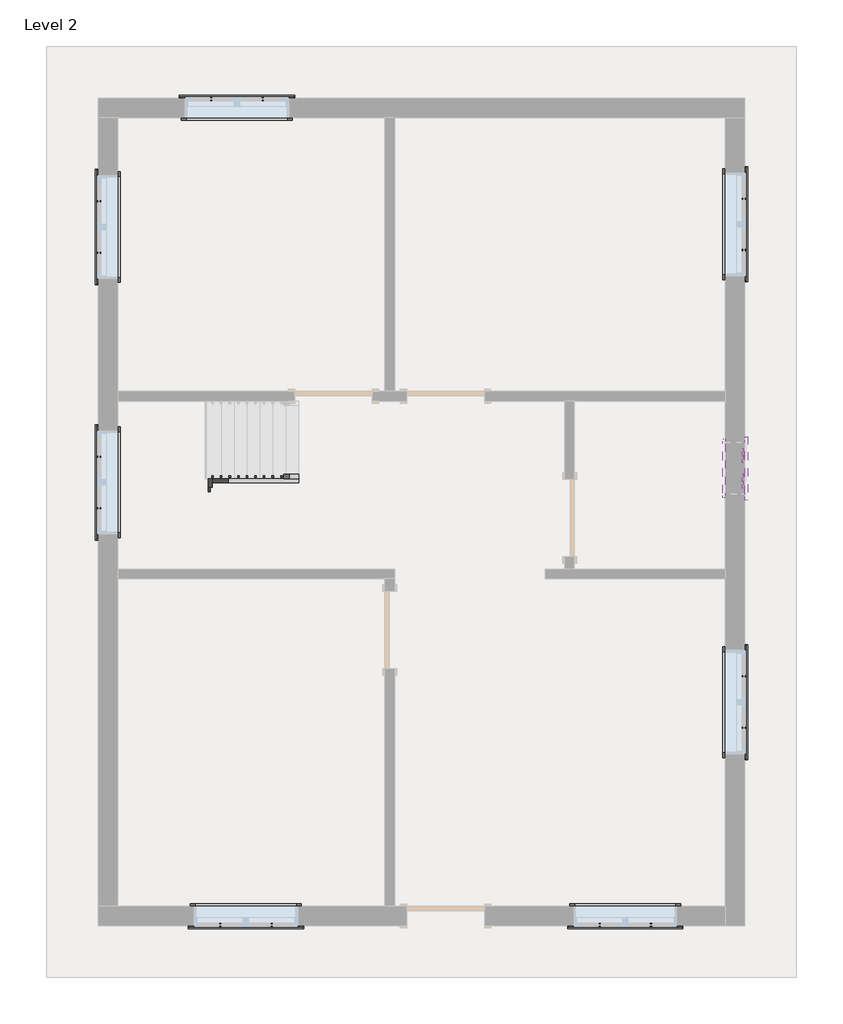
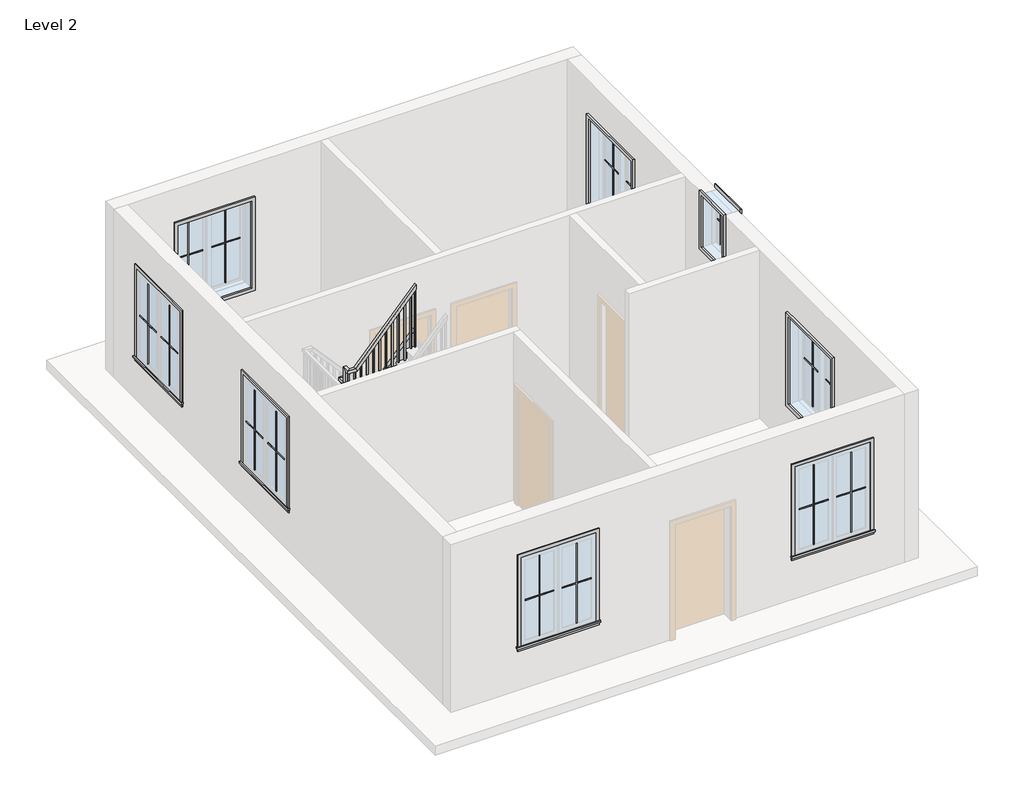
# One storey, part 2 of 2: 32 proxies, 3 members, 1 railing.
"""IFC4 building model written with IfcOpenShell, lengths in millimetres."""

from ifc_helpers import new_model, si_unit, frame, origin, place, context, project, spatial, polyline, outline, extrude, faceted_brep, transform, mapped, element, save
from components import muntin_pattern_2x2_muntin_pattern_2x2_6dad3731, muntin_pattern_2x2_muntin_pattern_2x2_a30a3345, muntin_pattern_2x2_muntin_pattern_2x2_53152e2c, muntin_pattern_2x2_muntin_pattern_2x2_e8f3e573, trim_window_exterior_flat_with_sill_92b9b949, trim_window_exterior_flat_with_sill_a665a915, trim_window_interior_flat_picture_frame_3bb882cf, trim_window_interior_flat_picture_frame_d485c387

model = new_model("IFC4")

# Units and contexts
model_context = context("Model", 3, world=origin())
ifc_project = project(units=[si_unit("LENGTHUNIT", "METRE", prefix="MILLI")], contexts=[model_context])

# Site, building, storey
site = spatial("IfcSite", under=ifc_project)
building = spatial("IfcBuilding", under=site)
storey = spatial("IfcBuildingStorey", under=building, Name="Level 2", Elevation=3048.0)

# Proxies
placement = place(None, origin())
muntin_pattern_2x2_muntin_pattern_2x2_shape = muntin_pattern_2x2_muntin_pattern_2x2_6dad3731(model_context)
element("IfcBuildingElementProxy", 1, Name="Muntin Pattern_2x2 : Muntin Pattern_2x2", ObjectType="Muntin Pattern_2x2 : Muntin Pattern_2x2", at=placement, inside=storey, context=model_context, shape_type="MappedRepresentation", body=[
    mapped(muntin_pattern_2x2_muntin_pattern_2x2_shape, transform((7785.1, 4733.925, 4032.25), x_axis=(-1.0, 0.0, 0.0), y_axis=(0.0, -1.0, 0.0), z_axis=(0.0, 0.0, 1.0))),
])
element("IfcBuildingElementProxy", 2, Name="Muntin Pattern_2x2 : Muntin Pattern_2x2", ObjectType="Muntin Pattern_2x2 : Muntin Pattern_2x2", at=placement, inside=storey, context=model_context, shape_type="MappedRepresentation", body=[
    mapped(muntin_pattern_2x2_muntin_pattern_2x2_shape, transform((3313.1125, 4733.925, 4032.25), x_axis=(-1.0, 0.0, 0.0), y_axis=(0.0, -1.0, 0.0), z_axis=(0.0, 0.0, 1.0))),
])
element("IfcBuildingElementProxy", 3, Name="Muntin Pattern_2x2 : Muntin Pattern_2x2", ObjectType="Muntin Pattern_2x2 : Muntin Pattern_2x2", at=placement, inside=storey, context=model_context, shape_type="MappedRepresentation", body=[
    mapped(muntin_pattern_2x2_muntin_pattern_2x2_shape, transform((8880.475, 13295.3125, 4032.25), x_axis=(0.0, -1.0, 0.0), y_axis=(1.0, 0.0, 0.0), z_axis=(0.0, 0.0, 1.0))),
])
element("IfcBuildingElementProxy", 4, Name="Muntin Pattern_2x2 : Muntin Pattern_2x2", ObjectType="Muntin Pattern_2x2 : Muntin Pattern_2x2", at=placement, inside=storey, context=model_context, shape_type="MappedRepresentation", body=[
    mapped(muntin_pattern_2x2_muntin_pattern_2x2_shape, transform((8880.475, 7662.8625, 4032.25), x_axis=(0.0, -1.0, 0.0), y_axis=(1.0, 0.0, 0.0), z_axis=(0.0, 0.0, 1.0))),
])
element("IfcBuildingElementProxy", 5, Name="Muntin Pattern_2x2 : Muntin Pattern_2x2", ObjectType="Muntin Pattern_2x2 : Muntin Pattern_2x2", at=placement, inside=storey, context=model_context, shape_type="MappedRepresentation", body=[
    mapped(muntin_pattern_2x2_muntin_pattern_2x2_shape, transform((1279.525, 12657.1375, 4032.25), x_axis=(0.0, 1.0, 0.0), y_axis=(-1.0, 0.0, 0.0), z_axis=(0.0, 0.0, 1.0))),
])
element("IfcBuildingElementProxy", 6, Name="Muntin Pattern_2x2 : Muntin Pattern_2x2", ObjectType="Muntin Pattern_2x2 : Muntin Pattern_2x2", at=placement, inside=storey, context=model_context, shape_type="MappedRepresentation", body=[
    mapped(muntin_pattern_2x2_muntin_pattern_2x2_shape, transform((1279.525, 9647.2375, 4032.25), x_axis=(0.0, 1.0, 0.0), y_axis=(-1.0, 0.0, 0.0), z_axis=(0.0, 0.0, 1.0))),
])
element("IfcBuildingElementProxy", 7, Name="Muntin Pattern_2x2 : Muntin Pattern_2x2", ObjectType="Muntin Pattern_2x2 : Muntin Pattern_2x2", at=placement, inside=storey, context=model_context, shape_type="MappedRepresentation", body=[
    mapped(muntin_pattern_2x2_muntin_pattern_2x2_shape, transform((2601.9125, 14468.475, 4032.25), x_axis=(1.0, 0.0, 0.0), y_axis=(0.0, 1.0, 0.0), z_axis=(0.0, 0.0, 1.0))),
])
muntin_pattern_2x2_muntin_pattern_2x2_2_shape = muntin_pattern_2x2_muntin_pattern_2x2_a30a3345(model_context)
element("IfcBuildingElementProxy", 8, Name="Muntin Pattern_2x2 : Muntin Pattern_2x2", ObjectType="Muntin Pattern_2x2 : Muntin Pattern_2x2", at=placement, inside=storey, context=model_context, shape_type="MappedRepresentation", body=[
    mapped(muntin_pattern_2x2_muntin_pattern_2x2_2_shape, transform((7178.675, 4733.925, 4032.25), x_axis=(1.0, 0.0, 0.0), y_axis=(0.0, 1.0, 0.0), z_axis=(0.0, 0.0, 1.0))),
])
element("IfcBuildingElementProxy", 9, Name="Muntin Pattern_2x2 : Muntin Pattern_2x2", ObjectType="Muntin Pattern_2x2 : Muntin Pattern_2x2", at=placement, inside=storey, context=model_context, shape_type="MappedRepresentation", body=[
    mapped(muntin_pattern_2x2_muntin_pattern_2x2_2_shape, transform((2706.6875, 4733.925, 4032.25), x_axis=(1.0, 0.0, 0.0), y_axis=(0.0, 1.0, 0.0), z_axis=(0.0, 0.0, 1.0))),
])
element("IfcBuildingElementProxy", 10, Name="Muntin Pattern_2x2 : Muntin Pattern_2x2", ObjectType="Muntin Pattern_2x2 : Muntin Pattern_2x2", at=placement, inside=storey, context=model_context, shape_type="MappedRepresentation", body=[
    mapped(muntin_pattern_2x2_muntin_pattern_2x2_2_shape, transform((8880.475, 12688.8875, 4032.25), x_axis=(0.0, 1.0, 0.0), y_axis=(-1.0, 0.0, 0.0), z_axis=(0.0, 0.0, 1.0))),
])
element("IfcBuildingElementProxy", 11, Name="Muntin Pattern_2x2 : Muntin Pattern_2x2", ObjectType="Muntin Pattern_2x2 : Muntin Pattern_2x2", at=placement, inside=storey, context=model_context, shape_type="MappedRepresentation", body=[
    mapped(muntin_pattern_2x2_muntin_pattern_2x2_2_shape, transform((8880.475, 7056.4375, 4032.25), x_axis=(0.0, 1.0, 0.0), y_axis=(-1.0, 0.0, 0.0), z_axis=(0.0, 0.0, 1.0))),
])
element("IfcBuildingElementProxy", 12, Name="Muntin Pattern_2x2 : Muntin Pattern_2x2", ObjectType="Muntin Pattern_2x2 : Muntin Pattern_2x2", at=placement, inside=storey, context=model_context, shape_type="MappedRepresentation", body=[
    mapped(muntin_pattern_2x2_muntin_pattern_2x2_2_shape, transform((1279.525, 13263.5625, 4032.25), x_axis=(0.0, -1.0, 0.0), y_axis=(1.0, 0.0, 0.0), z_axis=(0.0, 0.0, 1.0))),
])
element("IfcBuildingElementProxy", 13, Name="Muntin Pattern_2x2 : Muntin Pattern_2x2", ObjectType="Muntin Pattern_2x2 : Muntin Pattern_2x2", at=placement, inside=storey, context=model_context, shape_type="MappedRepresentation", body=[
    mapped(muntin_pattern_2x2_muntin_pattern_2x2_2_shape, transform((1279.525, 10253.6625, 4032.25), x_axis=(0.0, -1.0, 0.0), y_axis=(1.0, 0.0, 0.0), z_axis=(0.0, 0.0, 1.0))),
])
element("IfcBuildingElementProxy", 14, Name="Muntin Pattern_2x2 : Muntin Pattern_2x2", ObjectType="Muntin Pattern_2x2 : Muntin Pattern_2x2", at=placement, inside=storey, context=model_context, shape_type="MappedRepresentation", body=[
    mapped(muntin_pattern_2x2_muntin_pattern_2x2_2_shape, transform((3208.3375, 14468.475, 4032.25), x_axis=(-1.0, 0.0, 0.0), y_axis=(0.0, -1.0, 0.0), z_axis=(0.0, 0.0, 1.0))),
])
muntin_pattern_2x2_muntin_pattern_2x2_3_shape = muntin_pattern_2x2_muntin_pattern_2x2_53152e2c(model_context)
element("IfcBuildingElementProxy", 15, Name="Muntin Pattern_2x2 : Muntin Pattern_2x2", ObjectType="Muntin Pattern_2x2 : Muntin Pattern_2x2", at=placement, inside=storey, context=model_context, shape_type="MappedRepresentation", body=[
    mapped(muntin_pattern_2x2_muntin_pattern_2x2_3_shape, transform((8880.475, 10266.3625, 5251.45), x_axis=(0.0, -1.0, 0.0), y_axis=(1.0, 0.0, 0.0), z_axis=(0.0, 0.0, 1.0))),
])
muntin_pattern_2x2_muntin_pattern_2x2_4_shape = muntin_pattern_2x2_muntin_pattern_2x2_e8f3e573(model_context)
element("IfcBuildingElementProxy", 16, Name="Muntin Pattern_2x2 : Muntin Pattern_2x2", ObjectType="Muntin Pattern_2x2 : Muntin Pattern_2x2", at=placement, inside=storey, context=model_context, shape_type="MappedRepresentation", body=[
    mapped(muntin_pattern_2x2_muntin_pattern_2x2_4_shape, transform((8880.475, 9964.7375, 5251.45), x_axis=(0.0, 1.0, 0.0), y_axis=(-1.0, 0.0, 0.0), z_axis=(0.0, 0.0, 1.0))),
])
trim_window_exterior_flat_with_sill_shape = trim_window_exterior_flat_with_sill_92b9b949(model_context)
element("IfcBuildingElementProxy", 17, Name="Trim-Window-Exterior-Flat : with Sill", ObjectType="Trim-Window-Exterior-Flat : with Sill", at=placement, inside=storey, context=model_context, shape_type="MappedRepresentation", body=[
    mapped(trim_window_exterior_flat_with_sill_shape, transform((7481.8875, 4724.4, 5486.4), x_axis=(1.0, 0.0, 0.0), y_axis=(0.0, 0.0, 1.0), z_axis=(0.0, -1.0, 0.0))),
])
element("IfcBuildingElementProxy", 18, Name="Trim-Window-Exterior-Flat : with Sill", ObjectType="Trim-Window-Exterior-Flat : with Sill", at=placement, inside=storey, context=model_context, shape_type="MappedRepresentation", body=[
    mapped(trim_window_exterior_flat_with_sill_shape, transform((3009.9, 4724.4, 5486.4), x_axis=(1.0, 0.0, 0.0), y_axis=(0.0, 0.0, 1.0), z_axis=(0.0, -1.0, 0.0))),
])
element("IfcBuildingElementProxy", 19, Name="Trim-Window-Exterior-Flat : with Sill", ObjectType="Trim-Window-Exterior-Flat : with Sill", at=placement, inside=storey, context=model_context, shape_type="MappedRepresentation", body=[
    mapped(trim_window_exterior_flat_with_sill_shape, transform((8890.0, 12992.1, 5486.4), x_axis=(0.0, 1.0, 0.0), y_axis=(0.0, 0.0, 1.0), z_axis=(1.0, 0.0, 0.0))),
])
element("IfcBuildingElementProxy", 20, Name="Trim-Window-Exterior-Flat : with Sill", ObjectType="Trim-Window-Exterior-Flat : with Sill", at=placement, inside=storey, context=model_context, shape_type="MappedRepresentation", body=[
    mapped(trim_window_exterior_flat_with_sill_shape, transform((8890.0, 7359.65, 5486.4), x_axis=(0.0, 1.0, 0.0), y_axis=(0.0, 0.0, 1.0), z_axis=(1.0, 0.0, 0.0))),
])
element("IfcBuildingElementProxy", 21, Name="Trim-Window-Exterior-Flat : with Sill", ObjectType="Trim-Window-Exterior-Flat : with Sill", at=placement, inside=storey, context=model_context, shape_type="MappedRepresentation", body=[
    mapped(trim_window_exterior_flat_with_sill_shape, transform((1270.0, 12960.35, 5486.4), x_axis=(0.0, -1.0, 0.0), y_axis=(0.0, 0.0, 1.0), z_axis=(-1.0, 0.0, 0.0))),
])
element("IfcBuildingElementProxy", 22, Name="Trim-Window-Exterior-Flat : with Sill", ObjectType="Trim-Window-Exterior-Flat : with Sill", at=placement, inside=storey, context=model_context, shape_type="MappedRepresentation", body=[
    mapped(trim_window_exterior_flat_with_sill_shape, transform((1270.0, 9950.45, 5486.4), x_axis=(0.0, -1.0, 0.0), y_axis=(0.0, 0.0, 1.0), z_axis=(-1.0, 0.0, 0.0))),
])
element("IfcBuildingElementProxy", 23, Name="Trim-Window-Exterior-Flat : with Sill", ObjectType="Trim-Window-Exterior-Flat : with Sill", at=placement, inside=storey, context=model_context, shape_type="MappedRepresentation", body=[
    mapped(trim_window_exterior_flat_with_sill_shape, transform((2905.125, 14478.0, 5486.4), x_axis=(-1.0, 0.0, 0.0), y_axis=(0.0, 0.0, 1.0), z_axis=(0.0, 1.0, 0.0))),
])
trim_window_exterior_flat_with_sill_2_shape = trim_window_exterior_flat_with_sill_a665a915(model_context)
element("IfcBuildingElementProxy", 24, Name="Trim-Window-Exterior-Flat : with Sill", ObjectType="Trim-Window-Exterior-Flat : with Sill", at=placement, inside=storey, context=model_context, shape_type="MappedRepresentation", body=[
    mapped(trim_window_exterior_flat_with_sill_2_shape, transform((8890.0, 10115.55, 6096.0), x_axis=(0.0, 1.0, 0.0), y_axis=(0.0, 0.0, 1.0), z_axis=(1.0, 0.0, 0.0))),
])
trim_window_interior_flat_picture_frame_shape = trim_window_interior_flat_picture_frame_3bb882cf(model_context)
element("IfcBuildingElementProxy", 25, Name="Trim-Window-Interior-Flat : Picture Frame", ObjectType="Trim-Window-Interior-Flat : Picture Frame", at=placement, inside=storey, context=model_context, shape_type="MappedRepresentation", body=[
    mapped(trim_window_interior_flat_picture_frame_shape, transform((7481.8875, 4953.0, 5486.4), x_axis=(-1.0, 0.0, 0.0), y_axis=(0.0, 0.0, 1.0), z_axis=(0.0, 1.0, 0.0))),
])
element("IfcBuildingElementProxy", 26, Name="Trim-Window-Interior-Flat : Picture Frame", ObjectType="Trim-Window-Interior-Flat : Picture Frame", at=placement, inside=storey, context=model_context, shape_type="MappedRepresentation", body=[
    mapped(trim_window_interior_flat_picture_frame_shape, transform((3009.9, 4953.0, 5486.4), x_axis=(-1.0, 0.0, 0.0), y_axis=(0.0, 0.0, 1.0), z_axis=(0.0, 1.0, 0.0))),
])
element("IfcBuildingElementProxy", 27, Name="Trim-Window-Interior-Flat : Picture Frame", ObjectType="Trim-Window-Interior-Flat : Picture Frame", at=placement, inside=storey, context=model_context, shape_type="MappedRepresentation", body=[
    mapped(trim_window_interior_flat_picture_frame_shape, transform((8661.4, 12992.1, 5486.4), x_axis=(0.0, -1.0, 0.0), y_axis=(0.0, 0.0, 1.0), z_axis=(-1.0, 0.0, 0.0))),
])
element("IfcBuildingElementProxy", 28, Name="Trim-Window-Interior-Flat : Picture Frame", ObjectType="Trim-Window-Interior-Flat : Picture Frame", at=placement, inside=storey, context=model_context, shape_type="MappedRepresentation", body=[
    mapped(trim_window_interior_flat_picture_frame_shape, transform((8661.4, 7359.65, 5486.4), x_axis=(0.0, -1.0, 0.0), y_axis=(0.0, 0.0, 1.0), z_axis=(-1.0, 0.0, 0.0))),
])
element("IfcBuildingElementProxy", 29, Name="Trim-Window-Interior-Flat : Picture Frame", ObjectType="Trim-Window-Interior-Flat : Picture Frame", at=placement, inside=storey, context=model_context, shape_type="MappedRepresentation", body=[
    mapped(trim_window_interior_flat_picture_frame_shape, transform((1498.6, 12960.35, 5486.4), x_axis=(0.0, 1.0, 0.0), y_axis=(0.0, 0.0, 1.0), z_axis=(1.0, 0.0, 0.0))),
])
element("IfcBuildingElementProxy", 30, Name="Trim-Window-Interior-Flat : Picture Frame", ObjectType="Trim-Window-Interior-Flat : Picture Frame", at=placement, inside=storey, context=model_context, shape_type="MappedRepresentation", body=[
    mapped(trim_window_interior_flat_picture_frame_shape, transform((1498.6, 9950.45, 5486.4), x_axis=(0.0, 1.0, 0.0), y_axis=(0.0, 0.0, 1.0), z_axis=(1.0, 0.0, 0.0))),
])
element("IfcBuildingElementProxy", 31, Name="Trim-Window-Interior-Flat : Picture Frame", ObjectType="Trim-Window-Interior-Flat : Picture Frame", at=placement, inside=storey, context=model_context, shape_type="MappedRepresentation", body=[
    mapped(trim_window_interior_flat_picture_frame_shape, transform((2905.125, 14249.4, 5486.4), x_axis=(1.0, 0.0, 0.0), y_axis=(0.0, 0.0, 1.0), z_axis=(0.0, -1.0, 0.0))),
])
trim_window_interior_flat_picture_frame_2_shape = trim_window_interior_flat_picture_frame_d485c387(model_context)
element("IfcBuildingElementProxy", 32, Name="Trim-Window-Interior-Flat : Picture Frame", ObjectType="Trim-Window-Interior-Flat : Picture Frame", at=placement, inside=storey, context=model_context, shape_type="MappedRepresentation", body=[
    mapped(trim_window_interior_flat_picture_frame_2_shape, transform((8661.4, 10115.55, 6096.0), x_axis=(0.0, -1.0, 0.0), y_axis=(0.0, 0.0, 1.0), z_axis=(-1.0, 0.0, 0.0))),
])

# Members
element("IfcMember", 33, ObjectType="Stringer - 2\" Width", at=placement, inside=storey, context=model_context, shape_type="SweptSolid", body=[
    extrude(outline(polyline([(3048.0, 3632.2), (3322.6288314, 3632.2), (4451.5177203, 2616.2), (3995.8883192, 2616.2), (3048.0, 3469.2994873), (3048.0, 3632.2)])), frame((0.0, 9944.1, 0.0), z_axis=(0.0, 1.0, 0.0), x_axis=(0.0, 0.0, 1.0)), (0.0, 0.0, 1.0), 50.8),
])
element("IfcMember", 34, ObjectType="Stringer - 2\" Width", at=placement, inside=storey, context=model_context, shape_type="SweptSolid", body=[
    extrude(outline(polyline([(2565.4, 9994.9), (2616.2, 9994.9), (2616.2, 9893.3), (2565.4, 9893.3), (2565.4, 9994.9)])), frame((0.0, 0.0, 4174.0666667), z_axis=(0.0, 0.0, 1.0), x_axis=(1.0, 0.0, 0.0)), (0.0, 0.0, 1.0), 304.8),
])
element("IfcMember", 35, ObjectType="Stringer - 2\" Width", at=placement, inside=storey, context=model_context, shape_type="SweptSolid", body=[
    extrude(outline(polyline([(4677.2954981, 2565.4), (4221.666097, 2565.4), (5406.9994303, 3632.2), (5862.6288314, 3632.2), (4677.2954981, 2565.4)])), frame((0.0, 9842.5, 0.0), z_axis=(0.0, 1.0, 0.0), x_axis=(0.0, 0.0, 1.0)), (0.0, 0.0, 1.0), 50.8),
])

# Railing
element("IfcRailing", 36, ObjectType="Handrail - Rectangular", at=placement, inside=storey, context=model_context, shape_type="SolidModel", body=[
    faceted_brep([(3632.2, 9994.9, 4131.7333333), (3632.2, 9994.9, 4055.7950998), (3632.2, 10045.7, 4055.7950998), (3632.2, 10045.7, 4131.7333333), (2641.6, 9994.9, 5232.4), (2590.8, 9994.9, 5212.9062109), (2590.8, 10045.7, 5212.9062109), (2641.6, 10045.7, 5232.4), (2641.6, 9994.9, 5317.0666667), (2590.8, 9994.9, 5266.2666667), (2590.8, 10045.7, 5266.2666667), (2641.6, 10045.7, 5317.0666667), (2565.4, 9994.9, 5317.0666667), (2565.4, 9994.9, 5266.2666667), (2514.6, 10045.7, 5266.2666667), (2514.6, 10045.7, 5317.0666667), (2565.4, 9918.7, 5317.0666667), (2565.4, 9867.9, 5266.2666667), (2514.6, 9867.9, 5266.2666667), (2514.6, 9918.7, 5317.0666667), (2565.4, 9918.7, 5571.0666667), (2565.4, 9867.9, 5520.2666667), (2514.6, 9867.9, 5520.2666667), (2514.6, 9918.7, 5571.0666667), (2565.4, 9842.5, 5571.0666667), (2565.4, 9842.5, 5520.2666667), (2514.6, 9791.7, 5520.2666667), (2514.6, 9791.7, 5571.0666667), (2641.6, 9842.5, 5571.0666667), (2664.2244102, 9842.5, 5520.2666667), (2664.2244102, 9791.7, 5520.2666667), (2641.6, 9791.7, 5571.0666667), (3632.2, 9842.5, 6671.7333333), (3632.2, 9791.7, 6671.7333333), (3632.2, 9791.7, 6595.7950998), (3632.2, 9842.5, 6595.7950998)], [[[0, 1, 2, 3]], [[1, 0, 4, 5]], [[2, 1, 5, 6]], [[3, 2, 6, 7]], [[0, 3, 7, 4]], [[5, 4, 8, 9]], [[6, 5, 9, 10]], [[7, 6, 10, 11]], [[4, 7, 11, 8]], [[9, 8, 12, 13]], [[10, 9, 13, 14]], [[11, 10, 14, 15]], [[8, 11, 15, 12]], [[13, 12, 16, 17]], [[14, 13, 17, 18]], [[15, 14, 18, 19]], [[12, 15, 19, 16]], [[17, 16, 20, 21]], [[18, 17, 21, 22]], [[19, 18, 22, 23]], [[16, 19, 23, 20]], [[21, 20, 24, 25]], [[22, 21, 25, 26]], [[23, 22, 26, 27]], [[20, 23, 27, 24]], [[25, 24, 28, 29]], [[26, 25, 29, 30]], [[27, 26, 30, 31]], [[24, 27, 31, 28]], [[32, 33, 34, 35]], [[29, 28, 32, 35]], [[30, 29, 35, 34]], [[31, 30, 34, 33]], [[28, 31, 33, 32]]]),
    extrude(outline(polyline([(6500.5450998, 3546.475), (5588.0, 3546.475), (5588.0, 3565.525), (6521.7117665, 3565.525), (6500.5450998, 3546.475)])), frame((0.0, 9807.575, 0.0), z_axis=(0.0, 1.0, 0.0), x_axis=(0.0, 0.0, 1.0)), (0.0, 0.0, 1.0), 19.05),
    extrude(outline(polyline([(6387.6562109, 3444.875), (5418.6666667, 3444.875), (5418.6666667, 3463.925), (6408.8228776, 3463.925), (6387.6562109, 3444.875)])), frame((0.0, 9807.575, 0.0), z_axis=(0.0, 1.0, 0.0), x_axis=(0.0, 0.0, 1.0)), (0.0, 0.0, 1.0), 19.05),
    extrude(outline(polyline([(6274.767322, 3343.275), (5418.6666667, 3343.275), (5418.6666667, 3362.325), (6295.9339887, 3362.325), (6274.767322, 3343.275)])), frame((0.0, 9807.575, 0.0), z_axis=(0.0, 1.0, 0.0), x_axis=(0.0, 0.0, 1.0)), (0.0, 0.0, 1.0), 19.05),
    extrude(outline(polyline([(6161.8784332, 3241.675), (5249.3333333, 3241.675), (5249.3333333, 3260.725), (6183.0450998, 3260.725), (6161.8784332, 3241.675)])), frame((0.0, 9807.575, 0.0), z_axis=(0.0, 1.0, 0.0), x_axis=(0.0, 0.0, 1.0)), (0.0, 0.0, 1.0), 19.05),
    extrude(outline(polyline([(6048.9895443, 3140.075), (5080.0, 3140.075), (5080.0, 3159.125), (6070.1562109, 3159.125), (6048.9895443, 3140.075)])), frame((0.0, 9807.575, 0.0), z_axis=(0.0, 1.0, 0.0), x_axis=(0.0, 0.0, 1.0)), (0.0, 0.0, 1.0), 19.05),
    extrude(outline(polyline([(5936.1006554, 3038.475), (5080.0, 3038.475), (5080.0, 3057.525), (5957.267322, 3057.525), (5936.1006554, 3038.475)])), frame((0.0, 9807.575, 0.0), z_axis=(0.0, 1.0, 0.0), x_axis=(0.0, 0.0, 1.0)), (0.0, 0.0, 1.0), 19.05),
    extrude(outline(polyline([(5823.2117665, 2936.875), (4910.6666667, 2936.875), (4910.6666667, 2955.925), (5844.3784332, 2955.925), (5823.2117665, 2936.875)])), frame((0.0, 9807.575, 0.0), z_axis=(0.0, 1.0, 0.0), x_axis=(0.0, 0.0, 1.0)), (0.0, 0.0, 1.0), 19.05),
    extrude(outline(polyline([(5710.3228776, 2835.275), (4741.3333333, 2835.275), (4741.3333333, 2854.325), (5731.4895443, 2854.325), (5710.3228776, 2835.275)])), frame((0.0, 9807.575, 0.0), z_axis=(0.0, 1.0, 0.0), x_axis=(0.0, 0.0, 1.0)), (0.0, 0.0, 1.0), 19.05),
    extrude(outline(polyline([(5597.4339887, 2733.675), (4741.3333333, 2733.675), (4741.3333333, 2752.725), (5618.6006554, 2752.725), (5597.4339887, 2733.675)])), frame((0.0, 9807.575, 0.0), z_axis=(0.0, 1.0, 0.0), x_axis=(0.0, 0.0, 1.0)), (0.0, 0.0, 1.0), 19.05),
    extrude(outline(polyline([(5484.5450998, 2632.075), (4572.0, 2632.075), (4572.0, 2651.125), (5505.7117665, 2651.125), (5484.5450998, 2632.075)])), frame((0.0, 9807.575, 0.0), z_axis=(0.0, 1.0, 0.0), x_axis=(0.0, 0.0, 1.0)), (0.0, 0.0, 1.0), 19.05),
    extrude(outline(polyline([(2549.525, 9928.225), (2549.525, 9909.175), (2530.475, 9909.175), (2530.475, 9928.225), (2549.525, 9928.225)])), frame((0.0, 0.0, 4402.6666667), z_axis=(0.0, 0.0, 1.0), x_axis=(1.0, 0.0, 0.0)), (0.0, 0.0, 1.0), 863.6),
    extrude(outline(polyline([(2625.725, 10010.775), (2606.675, 10010.775), (2606.675, 10029.825), (2625.725, 10029.825), (2625.725, 10010.775)])), frame((0.0, 0.0, 4233.3333333), z_axis=(0.0, 0.0, 1.0), x_axis=(1.0, 0.0, 0.0)), (0.0, 0.0, 1.0), 1032.9333333),
    extrude(outline(polyline([(5082.3784332, 2708.275), (4233.3333333, 2708.275), (4233.3333333, 2727.325), (5061.2117665, 2727.325), (5082.3784332, 2708.275)])), frame((0.0, 10010.775, 0.0), z_axis=(0.0, 1.0, 0.0), x_axis=(0.0, 0.0, 1.0)), (0.0, 0.0, 1.0), 19.05),
    extrude(outline(polyline([(4969.4895443, 2809.875), (4064.0, 2809.875), (4064.0, 2828.925), (4948.3228776, 2828.925), (4969.4895443, 2809.875)])), frame((0.0, 10010.775, 0.0), z_axis=(0.0, 1.0, 0.0), x_axis=(0.0, 0.0, 1.0)), (0.0, 0.0, 1.0), 19.05),
    extrude(outline(polyline([(4856.6006554, 2911.475), (3894.6666667, 2911.475), (3894.6666667, 2930.525), (4835.4339887, 2930.525), (4856.6006554, 2911.475)])), frame((0.0, 10010.775, 0.0), z_axis=(0.0, 1.0, 0.0), x_axis=(0.0, 0.0, 1.0)), (0.0, 0.0, 1.0), 19.05),
    extrude(outline(polyline([(4743.7117665, 3013.075), (3894.6666667, 3013.075), (3894.6666667, 3032.125), (4722.5450998, 3032.125), (4743.7117665, 3013.075)])), frame((0.0, 10010.775, 0.0), z_axis=(0.0, 1.0, 0.0), x_axis=(0.0, 0.0, 1.0)), (0.0, 0.0, 1.0), 19.05),
    extrude(outline(polyline([(4630.8228776, 3114.675), (3725.3333333, 3114.675), (3725.3333333, 3133.725), (4609.6562109, 3133.725), (4630.8228776, 3114.675)])), frame((0.0, 10010.775, 0.0), z_axis=(0.0, 1.0, 0.0), x_axis=(0.0, 0.0, 1.0)), (0.0, 0.0, 1.0), 19.05),
    extrude(outline(polyline([(4517.9339887, 3216.275), (3556.0, 3216.275), (3556.0, 3235.325), (4496.767322, 3235.325), (4517.9339887, 3216.275)])), frame((0.0, 10010.775, 0.0), z_axis=(0.0, 1.0, 0.0), x_axis=(0.0, 0.0, 1.0)), (0.0, 0.0, 1.0), 19.05),
    extrude(outline(polyline([(4405.0450998, 3317.875), (3556.0, 3317.875), (3556.0, 3336.925), (4383.8784332, 3336.925), (4405.0450998, 3317.875)])), frame((0.0, 10010.775, 0.0), z_axis=(0.0, 1.0, 0.0), x_axis=(0.0, 0.0, 1.0)), (0.0, 0.0, 1.0), 19.05),
    extrude(outline(polyline([(4292.1562109, 3419.475), (3386.6666667, 3419.475), (3386.6666667, 3438.525), (4270.9895443, 3438.525), (4292.1562109, 3419.475)])), frame((0.0, 10010.775, 0.0), z_axis=(0.0, 1.0, 0.0), x_axis=(0.0, 0.0, 1.0)), (0.0, 0.0, 1.0), 19.05),
    extrude(outline(polyline([(4179.267322, 3521.075), (3217.3333333, 3521.075), (3217.3333333, 3540.125), (4158.1006554, 3540.125), (4179.267322, 3521.075)])), frame((0.0, 10010.775, 0.0), z_axis=(0.0, 1.0, 0.0), x_axis=(0.0, 0.0, 1.0)), (0.0, 0.0, 1.0), 19.05),
    extrude(outline(polyline([(2549.525, 9826.625), (2549.525, 9807.575), (2530.475, 9807.575), (2530.475, 9826.625), (2549.525, 9826.625)])), frame((0.0, 0.0, 4402.6666667), z_axis=(0.0, 0.0, 1.0), x_axis=(1.0, 0.0, 0.0)), (0.0, 0.0, 1.0), 1117.6),
    extrude(outline(polyline([(2549.525, 10010.775), (2530.475, 10010.775), (2530.475, 10029.825), (2549.525, 10029.825), (2549.525, 10010.775)])), frame((0.0, 0.0, 4402.6666667), z_axis=(0.0, 0.0, 1.0), x_axis=(1.0, 0.0, 0.0)), (0.0, 0.0, 1.0), 863.6),
    extrude(outline(polyline([(6574.6284332, 3613.15), (5588.0, 3613.15), (5588.0, 3632.2), (6595.7950998, 3632.2), (6574.6284332, 3613.15)])), frame((0.0, 9807.575, 0.0), z_axis=(0.0, 1.0, 0.0), x_axis=(0.0, 0.0, 1.0)), (0.0, 0.0, 1.0), 19.05),
    extrude(outline(polyline([(4076.9617665, 3613.15), (3217.3333333, 3613.15), (3217.3333333, 3632.2), (4055.7950998, 3632.2), (4076.9617665, 3613.15)])), frame((0.0, 10010.775, 0.0), z_axis=(0.0, 1.0, 0.0), x_axis=(0.0, 0.0, 1.0)), (0.0, 0.0, 1.0), 19.05),
])

save(model, "model.ifc")

# Revit data of these elements
# Type "Muntin Pattern_2x2 : Muntin Pattern_2x2"
#   Width [instance default] = 4' - 0"
#   Thickness = 0' - 0 1/2"
#   Height [instance default] = 4' - 0"
#   Distance = 0' - 0 3/4"
#   Interior Material [instance default] = none
#   Exterior Material [instance default] = none
#   Default Elevation = 0
# Type "Trim-Window-Exterior-Flat : with Sill"
#   Trim Width = 0' - 2 1/4"
#   Trim Thickness_Picture Frame = 0' - 1 1/4"
#   Trim Thickness_with Sill = 0' - 0 3/4"
#   Sill Thickness = 0' - 1 1/4"
#   Opening Width [instance default] = 2' - 0"
#   Opening Height [instance default] = 3' - 0"
#   Default Elevation = 4' - 0"
#   Sill = yes
#   Picture Frame = no
#   Trim Material [instance default] = none
# Type "Trim-Window-Interior-Flat : Picture Frame"
#   Trim Thickness_Picture Frame = 0' - 1 1/4"
#   Trim Width = 0' - 2 1/4"
#   Trim Thickness_with Sill = 0' - 0 3/4"
#   Sill Thickness = 0' - 1 1/4"
#   Opening Width [instance default] = 2' - 0"
#   Opening Height [instance default] = 3' - 0"
#   Default Elevation = 4' - 0"
#   Sill = no
#   Picture Frame = yes
#   Trim Material [instance default] = none
# Type "Handrail - Rectangular"
#   Assembly Code = "C2010400"
#   built-in parameter 1008612 = 0.0416667 (stored number, unit not read)
#   built-in parameter 1008611 = 0.0416667 (stored number, unit not read)
#   built-in parameter 1008609 = 0.333333 (stored number, unit not read)
#   built-in parameter 1008604 = 0.166667 (stored number, unit not read)
#   built-in parameter 1008603 = 0.166667 (stored number, unit not read)
#   Railing Height = 3' - 0"
#   built-in parameter 1008630 = 2
#   built-in parameter 1008610 = 2
#   built-in parameter 1008618 = Baluster - Square : 3/4"
# Elements 1, 2, 3, 4, 5, 6, 7, 8, 9, 10, 11, 12, 13, 14 (IfcBuildingElementProxy, "Muntin Pattern_2x2 : Muntin Pattern_2x2")
#   Width = 1' - 6 5/8"
#   Height = 4' - 6 1/2"
#   Interior Material = Wood - Stained
#   Exterior Material = Clad - White
#   Phase Created = New Construction
#   Materials on its faces: "Clad - White", "Wood - Stained"
# Elements 15, 16 (IfcBuildingElementProxy, "Muntin Pattern_2x2 : Muntin Pattern_2x2")
#   Width = 0' - 6 5/8"
#   Height = 2' - 6 1/2"
#   Interior Material = Wood - Stained
#   Exterior Material = Clad - White
#   Phase Created = New Construction
#   Materials on its faces: "Clad - White", "Wood - Stained"
# Elements 17, 18, 19, 20, 21, 22, 23 (IfcBuildingElementProxy, "Trim-Window-Exterior-Flat : with Sill")
#   Opening Width = 4' - 0"
#   Opening Height = 5' - 0"
#   Trim Material = Clad - White
#   Phase Created = New Construction
#   Materials on its faces: "Clad - White"
# Element 24 (IfcBuildingElementProxy, "Trim-Window-Exterior-Flat : with Sill")
#   Opening Width = 2' - 0"
#   Opening Height = 3' - 0"
#   Trim Material = Clad - White
#   Phase Created = New Construction
#   Materials on its faces: "Clad - White"
# Elements 25, 26, 27, 28, 29, 30, 31 (IfcBuildingElementProxy, "Trim-Window-Interior-Flat : Picture Frame")
#   Opening Width = 4' - 0"
#   Opening Height = 5' - 0"
#   Trim Material = Wood - Stained
#   Phase Created = New Construction
#   Materials on its faces: "Wood - Stained"
# Element 32 (IfcBuildingElementProxy, "Trim-Window-Interior-Flat : Picture Frame")
#   Opening Width = 2' - 0"
#   Opening Height = 3' - 0"
#   Trim Material = Wood - Stained
#   Phase Created = New Construction
#   Materials on its faces: "Wood - Stained"
# Elements 33, 34, 35 (IfcMember, "Stringer - 2\" Width")
#   Phase Created = New Construction
# Element 36 (IfcRailing, "Handrail - Rectangular")
#   Phase Created = New Construction
# Materials
#   "Clad - White": class "Wood", colour RGB 242 242 238, transparency 0, Cost = 0
#   "Wood - Stained": class "Wood", colour RGB 224 178 126, transparency 0, Cost = 0
